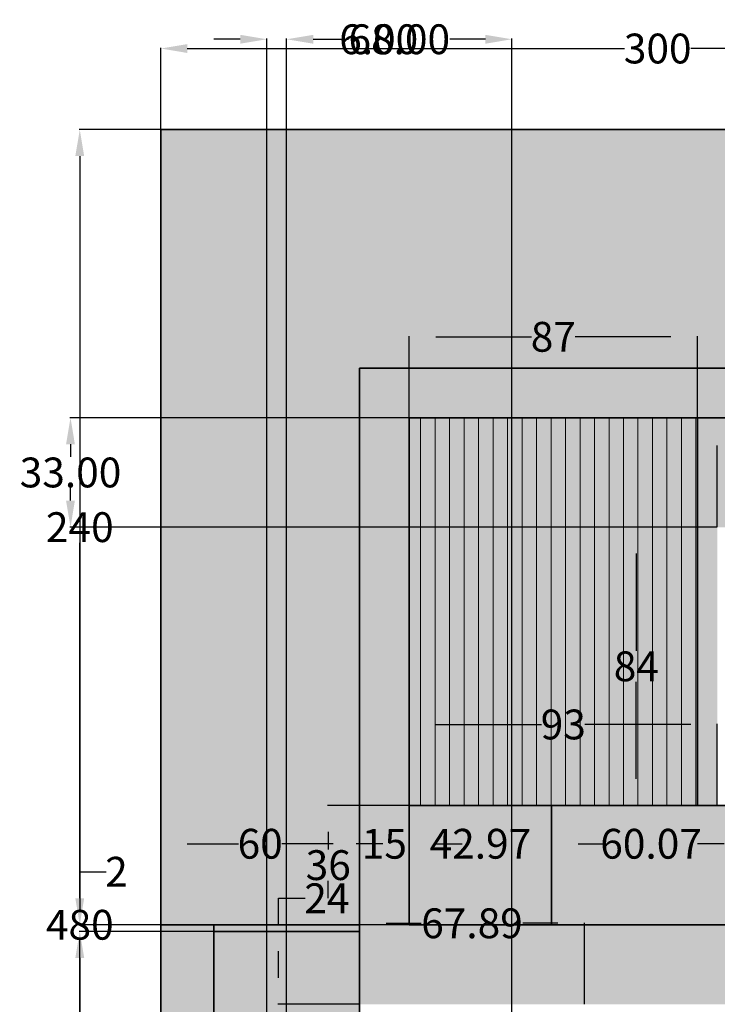
# Model space of a CAD drawing. Units: inches. Extents: x 207 to 609, y 30 to 576.
# Tile 3 of 4: x 207 to 418, y 279 to 576. Entities that reach past the tile are written whole.
import ezdxf

# ---------------------------------------------------------------- set-up
doc = ezdxf.new("R2010")
doc.units = ezdxf.units.IN
doc.header["$MEASUREMENT"] = 0
for name, color, linetype, lineweight in [('A-ANNO-DIMS', 2, 'Continuous', 18), ('A-ELEV', 7, 'Continuous', 35), ('A-ELEV-PATT', 251, 'Continuous', 13), ('A-ELEV-PATT-CLAD', 67, 'Continuous', 13), ('A-ELEV-PATT-WOOD', 19, 'Continuous', 13)]:
    doc.layers.add(name, color=color, linetype=linetype, lineweight=lineweight)
doc.styles.get("Standard").update_dxf_attribs({"font": 'arial.ttf'})
doc.dimstyles.get("Standard").update_dxf_attribs({"dimtxt": 9, "dimasz": 8, "dimexe": 0.18, "dimexo": 0.0625, "dimgap": 0.09, "dimtad": 0, "dimtih": 1, "dimtoh": 1, "dimdec": 0, "dimzin": 0, "dimdsep": 46, "dimlunit": 3, "dimtxsty": 'Standard', "dimcen": 0.09, "dimadec": 0, "dimazin": 0, "dimtfac": 1, "dimtdec": 0, "dimtofl": 0, "dimtmove": 0, "dimatfit": 3, "dimfxl": 1, "dimtolj": 1, "dimtzin": 0, "dimarcsym": 0})

# ---------------------------------------------------------------- blocks, each defined once
blk = doc.blocks.new('*D7')
at = {"layer": 'A-ANNO-DIMS', "color": 0, "lineweight": -2, "transparency": 16777216}
for p, q in [((249.7, 542.85), (249.7, 567.42)), ((257.7, 567.24), (389.68, 567.24)), ((541.7, 567.24), (409.71, 567.24)), ((549.7, 542.85), (549.7, 567.42))]:
    blk.add_line(p, q, dxfattribs=at)
at = {"layer": 'A-ANNO-DIMS', "color": 0, "transparency": 16777216}
for points in [[(257.7, 568.57), (257.7, 565.9), (249.7, 567.24)], [(541.7, 568.57), (541.7, 565.9), (549.7, 567.24)]]:
    blk.add_solid(points, dxfattribs=at)
at = {"layer": 'Defpoints', "color": 0, "transparency": 16777216}
for p in [(549.7, 567.24), (249.7, 542.79), (549.7, 542.79)]:
    blk.add_point(p, dxfattribs=at)
at = {"layer": 'A-ANNO-DIMS', "color": 0, "transparency": 16777216, "insert": (399.7, 567.24), "char_height": 9, "attachment_point": 5}
blk.add_mtext('\\A1;300', dxfattribs=at)
blk = doc.blocks.new('*D8')
at = {"layer": 'A-ANNO-DIMS', "color": 0, "lineweight": -2, "transparency": 16777216}
for p, q in [((249.63, 542.79), (225.07, 542.79)), ((225.25, 534.79), (225.25, 307.47)), ((225.25, 70.79), (225.25, 298.1)), ((249.63, 62.79), (225.07, 62.79))]:
    blk.add_line(p, q, dxfattribs=at)
at = {"layer": 'A-ANNO-DIMS', "color": 0, "transparency": 16777216}
for points in [[(223.91, 534.79), (226.58, 534.79), (225.25, 542.79)], [(223.91, 70.79), (226.58, 70.79), (225.25, 62.79)]]:
    blk.add_solid(points, dxfattribs=at)
at = {"layer": 'Defpoints', "color": 0, "transparency": 16777216}
for p in [(225.25, 542.79), (249.7, 542.79), (249.7, 62.79)]:
    blk.add_point(p, dxfattribs=at)
at = {"layer": 'A-ANNO-DIMS', "color": 0, "transparency": 16777216, "insert": (225.25, 302.79), "char_height": 9, "attachment_point": 5}
blk.add_mtext('\\A1;480', dxfattribs=at)
blk = doc.blocks.new('*D15')
at = {"layer": 'A-ANNO-DIMS', "color": 0, "lineweight": -2, "transparency": 16777216}
for p, q in [((265.63, 300.79), (225.07, 300.79)), ((225.25, 292.79), (225.25, 270.47)), ((225.25, 238.79), (225.25, 261.1)), ((265.63, 230.79), (225.07, 230.79))]:
    blk.add_line(p, q, dxfattribs=at)
at = {"layer": 'A-ANNO-DIMS', "color": 0, "transparency": 16777216}
for points in [[(223.91, 292.79), (226.58, 292.79), (225.25, 300.79)], [(223.91, 238.79), (226.58, 238.79), (225.25, 230.79)]]:
    blk.add_solid(points, dxfattribs=at)
at = {"layer": 'Defpoints', "color": 0, "transparency": 16777216}
for p in [(225.25, 300.79), (265.7, 300.79), (265.7, 230.79)]:
    blk.add_point(p, dxfattribs=at)
at = {"layer": 'A-ANNO-DIMS', "color": 0, "transparency": 16777216, "insert": (225.25, 265.79), "char_height": 9, "attachment_point": 5}
blk.add_mtext('\\A1;70', dxfattribs=at)
blk = doc.blocks.new('*D16')
at = {"layer": 'A-ANNO-DIMS', "color": 0, "lineweight": -2, "transparency": 16777216}
for p, q in [((225.25, 310.79), (225.25, 318.79)), ((225.25, 318.79), (233.25, 318.79)), ((265.63, 302.79), (225.07, 302.79)), ((265.63, 300.79), (225.07, 300.79)), ((225.25, 292.79), (225.25, 284.79))]:
    blk.add_line(p, q, dxfattribs=at)
at = {"layer": 'A-ANNO-DIMS', "color": 0, "transparency": 16777216}
for points in [[(223.91, 310.79), (226.58, 310.79), (225.25, 302.79)], [(223.91, 292.79), (226.58, 292.79), (225.25, 300.79)]]:
    blk.add_solid(points, dxfattribs=at)
at = {"layer": 'Defpoints', "color": 0, "transparency": 16777216}
for p in [(225.25, 302.79), (265.7, 302.79), (265.7, 300.79)]:
    blk.add_point(p, dxfattribs=at)
at = {"layer": 'A-ANNO-DIMS', "color": 0, "transparency": 16777216, "insert": (236.32, 318.79), "char_height": 9, "attachment_point": 5}
blk.add_mtext('\\A1;2', dxfattribs=at)
blk = doc.blocks.new('*D17')
at = {"layer": 'A-ANNO-DIMS', "color": 0, "lineweight": -2, "transparency": 16777216}
for p, q in [((249.63, 542.79), (225.07, 542.79)), ((225.25, 534.79), (225.25, 427.47)), ((225.25, 310.79), (225.25, 418.1)), ((249.63, 302.79), (225.07, 302.79))]:
    blk.add_line(p, q, dxfattribs=at)
at = {"layer": 'A-ANNO-DIMS', "color": 0, "transparency": 16777216}
for points in [[(223.91, 534.79), (226.58, 534.79), (225.25, 542.79)], [(223.91, 310.79), (226.58, 310.79), (225.25, 302.79)]]:
    blk.add_solid(points, dxfattribs=at)
at = {"layer": 'Defpoints', "color": 0, "transparency": 16777216}
for p in [(225.25, 542.79), (249.7, 542.79), (249.7, 302.79)]:
    blk.add_point(p, dxfattribs=at)
at = {"layer": 'A-ANNO-DIMS', "color": 0, "transparency": 16777216, "insert": (225.25, 422.79), "char_height": 9, "attachment_point": 5}
blk.add_mtext('\\A1;240', dxfattribs=at)
blk = doc.blocks.new('*D26')
at = {"layer": 'A-ANNO-DIMS', "color": 0, "lineweight": -2, "transparency": 16777216}
for p, q in [((285.25, 302.79), (285.25, 310.79)), ((285.25, 310.79), (293.25, 310.79)), ((309.63, 302.79), (285.07, 302.79)), ((285.25, 286.79), (285.25, 294.79)), ((309.63, 278.79), (285.07, 278.79))]:
    blk.add_line(p, q, dxfattribs=at)
at = {"layer": 'A-ANNO-DIMS', "color": 0, "transparency": 16777216}
for points in [[(283.91, 294.79), (286.58, 294.79), (285.25, 302.79)], [(283.91, 286.79), (286.58, 286.79), (285.25, 278.79)]]:
    blk.add_solid(points, dxfattribs=at)
at = {"layer": 'Defpoints', "color": 0, "transparency": 16777216}
for p in [(285.25, 302.79), (309.7, 302.79), (309.7, 278.79)]:
    blk.add_point(p, dxfattribs=at)
at = {"layer": 'A-ANNO-DIMS', "color": 0, "transparency": 16777216, "insert": (299.84, 310.79), "char_height": 9, "attachment_point": 5}
blk.add_mtext('\\A1;24', dxfattribs=at)
blk = doc.blocks.new('*D39')
at = {"layer": 'A-ANNO-DIMS', "color": 0, "lineweight": -2, "transparency": 16777216}
for p, q in [((249.7, 302.85), (249.7, 327.42)), ((257.7, 327.24), (273.15, 327.24)), ((301.7, 327.24), (286.24, 327.24)), ((309.7, 302.85), (309.7, 327.42))]:
    blk.add_line(p, q, dxfattribs=at)
at = {"layer": 'A-ANNO-DIMS', "color": 0, "transparency": 16777216}
for points in [[(257.7, 328.57), (257.7, 325.9), (249.7, 327.24)], [(301.7, 328.57), (301.7, 325.9), (309.7, 327.24)]]:
    blk.add_solid(points, dxfattribs=at)
at = {"layer": 'Defpoints', "color": 0, "transparency": 16777216}
for p in [(309.7, 327.24), (249.7, 302.79), (309.7, 302.79)]:
    blk.add_point(p, dxfattribs=at)
at = {"layer": 'A-ANNO-DIMS', "color": 0, "transparency": 16777216, "insert": (279.7, 327.24), "char_height": 9, "attachment_point": 5}
blk.add_mtext('\\A1;60', dxfattribs=at)
blk = doc.blocks.new('*D40')
at = {"layer": 'A-ANNO-DIMS', "color": 0, "lineweight": -2, "transparency": 16777216}
for p, q in [((301.7, 327.24), (293.7, 327.24)), ((309.7, 302.85), (309.7, 327.42)), ((324.7, 302.85), (324.7, 327.42)), ((332.7, 327.24), (340.7, 327.24))]:
    blk.add_line(p, q, dxfattribs=at)
at = {"layer": 'A-ANNO-DIMS', "color": 0, "transparency": 16777216}
for points in [[(301.7, 328.57), (301.7, 325.9), (309.7, 327.24)], [(332.7, 328.57), (332.7, 325.9), (324.7, 327.24)]]:
    blk.add_solid(points, dxfattribs=at)
at = {"layer": 'Defpoints', "color": 0, "transparency": 16777216}
for p in [(324.7, 327.24), (309.7, 302.79), (324.7, 302.79)]:
    blk.add_point(p, dxfattribs=at)
at = {"layer": 'A-ANNO-DIMS', "color": 0, "transparency": 16777216, "insert": (317.2, 327.24), "char_height": 9, "attachment_point": 5}
blk.add_mtext('\\A1;15', dxfattribs=at)
blk = doc.blocks.new('*D41')
at = {"layer": 'A-ANNO-DIMS', "color": 0, "lineweight": -2, "transparency": 16777216}
for p, q in [((324.7, 455.85), (324.7, 480.42)), ((332.7, 480.24), (361.65, 480.24)), ((403.7, 480.24), (374.74, 480.24)), ((411.7, 455.85), (411.7, 480.42))]:
    blk.add_line(p, q, dxfattribs=at)
at = {"layer": 'A-ANNO-DIMS', "color": 0, "transparency": 16777216}
for points in [[(332.7, 481.57), (332.7, 478.9), (324.7, 480.24)], [(403.7, 481.57), (403.7, 478.9), (411.7, 480.24)]]:
    blk.add_solid(points, dxfattribs=at)
at = {"layer": 'Defpoints', "color": 0, "transparency": 16777216}
for p in [(411.7, 480.24), (324.7, 455.79), (411.7, 455.79)]:
    blk.add_point(p, dxfattribs=at)
at = {"layer": 'A-ANNO-DIMS', "color": 0, "transparency": 16777216, "insert": (368.2, 480.24), "char_height": 9, "attachment_point": 5}
blk.add_mtext('\\A1;87', dxfattribs=at)
blk = doc.blocks.new('*D43')
at = {"layer": 'A-ANNO-DIMS', "color": 0, "lineweight": -2, "transparency": 16777216}
for p, q in [((324.7, 338.85), (324.7, 363.42)), ((332.7, 363.24), (364.66, 363.24)), ((409.7, 363.24), (377.73, 363.24)), ((417.7, 338.85), (417.7, 363.42))]:
    blk.add_line(p, q, dxfattribs=at)
at = {"layer": 'A-ANNO-DIMS', "color": 0, "transparency": 16777216}
for points in [[(332.7, 364.57), (332.7, 361.9), (324.7, 363.24)], [(409.7, 364.57), (409.7, 361.9), (417.7, 363.24)]]:
    blk.add_solid(points, dxfattribs=at)
at = {"layer": 'Defpoints', "color": 0, "transparency": 16777216}
for p in [(417.7, 363.24), (324.7, 338.79), (417.7, 338.79)]:
    blk.add_point(p, dxfattribs=at)
at = {"layer": 'A-ANNO-DIMS', "color": 0, "transparency": 16777216, "insert": (371.2, 363.24), "char_height": 9, "attachment_point": 5}
blk.add_mtext('\\A1;93', dxfattribs=at)
blk = doc.blocks.new('*D44')
at = {"layer": 'A-ANNO-DIMS', "color": 0, "lineweight": -2, "transparency": 16777216}
for p, q in [((417.7, 422.85), (417.7, 447.42)), ((425.7, 447.24), (438.18, 447.24)), ((463.7, 447.24), (451.21, 447.24)), ((471.7, 422.85), (471.7, 447.42))]:
    blk.add_line(p, q, dxfattribs=at)
at = {"layer": 'A-ANNO-DIMS', "color": 0, "transparency": 16777216}
for points in [[(425.7, 448.57), (425.7, 445.9), (417.7, 447.24)], [(463.7, 448.57), (463.7, 445.9), (471.7, 447.24)]]:
    blk.add_solid(points, dxfattribs=at)
at = {"layer": 'Defpoints', "color": 0, "transparency": 16777216}
for p in [(471.7, 447.24), (417.7, 422.79), (471.7, 422.79)]:
    blk.add_point(p, dxfattribs=at)
at = {"layer": 'A-ANNO-DIMS', "color": 0, "transparency": 16777216, "insert": (444.7, 447.24), "char_height": 9, "attachment_point": 5}
blk.add_mtext('\\A1;54', dxfattribs=at)
blk = doc.blocks.new('*D47')
at = {"layer": 'A-ANNO-DIMS', "color": 0, "lineweight": -2, "transparency": 16777216}
for p, q in [((316.7, 327.24), (308.7, 327.24)), ((324.7, 302.85), (324.7, 327.42)), ((367.66, 302.85), (367.66, 327.42)), ((375.66, 327.24), (383.66, 327.24))]:
    blk.add_line(p, q, dxfattribs=at)
at = {"layer": 'A-ANNO-DIMS', "color": 0, "transparency": 16777216}
for points in [[(316.7, 328.57), (316.7, 325.9), (324.7, 327.24)], [(375.66, 328.57), (375.66, 325.9), (367.66, 327.24)]]:
    blk.add_solid(points, dxfattribs=at)
at = {"layer": 'Defpoints', "color": 0, "transparency": 16777216}
for p in [(367.66, 327.24), (324.7, 302.79), (367.66, 302.79)]:
    blk.add_point(p, dxfattribs=at)
at = {"layer": 'A-ANNO-DIMS', "color": 0, "transparency": 16777216, "insert": (346.18, 327.24), "char_height": 9, "attachment_point": 5}
blk.add_mtext('\\A1;42.97', dxfattribs=at)
blk = doc.blocks.new('*D48')
at = {"layer": 'A-ANNO-DIMS', "color": 0, "lineweight": -2, "transparency": 16777216}
for p, q in [((367.66, 302.85), (367.66, 327.42)), ((375.66, 327.24), (382.4, 327.24)), ((419.73, 327.24), (413, 327.24)), ((427.73, 302.85), (427.73, 327.42))]:
    blk.add_line(p, q, dxfattribs=at)
at = {"layer": 'A-ANNO-DIMS', "color": 0, "transparency": 16777216}
for points in [[(375.66, 328.57), (375.66, 325.9), (367.66, 327.24)], [(419.73, 328.57), (419.73, 325.9), (427.73, 327.24)]]:
    blk.add_solid(points, dxfattribs=at)
at = {"layer": 'Defpoints', "color": 0, "transparency": 16777216}
for p in [(427.73, 327.24), (367.66, 302.79), (427.73, 302.79)]:
    blk.add_point(p, dxfattribs=at)
at = {"layer": 'A-ANNO-DIMS', "color": 0, "transparency": 16777216, "insert": (397.7, 327.24), "char_height": 9, "attachment_point": 5}
blk.add_mtext('\\A1;60.07', dxfattribs=at)
blk = doc.blocks.new('*D49')
at = {"layer": 'A-ANNO-DIMS', "color": 0, "lineweight": -2, "transparency": 16777216}
for p, q in [((419.73, 327.24), (411.73, 327.24)), ((427.73, 302.85), (427.73, 327.42)), ((459.05, 302.85), (459.05, 327.42)), ((467.05, 327.24), (475.05, 327.24))]:
    blk.add_line(p, q, dxfattribs=at)
at = {"layer": 'A-ANNO-DIMS', "color": 0, "transparency": 16777216}
for points in [[(419.73, 328.57), (419.73, 325.9), (427.73, 327.24)], [(467.05, 328.57), (467.05, 325.9), (459.05, 327.24)]]:
    blk.add_solid(points, dxfattribs=at)
at = {"layer": 'Defpoints', "color": 0, "transparency": 16777216}
for p in [(459.05, 327.24), (427.73, 302.79), (459.05, 302.79)]:
    blk.add_point(p, dxfattribs=at)
at = {"layer": 'A-ANNO-DIMS', "color": 0, "transparency": 16777216, "insert": (443.39, 327.24), "char_height": 9, "attachment_point": 5}
blk.add_mtext('\\A1;31.32', dxfattribs=at)
blk = doc.blocks.new('*D51')
at = {"layer": 'A-ANNO-DIMS', "color": 0, "lineweight": -2, "transparency": 16777216}
for p, q in [((324.63, 338.79), (300.07, 338.79)), ((300.25, 330.79), (300.25, 325.47)), ((300.25, 310.79), (300.25, 316.1)), ((324.63, 302.79), (300.07, 302.79))]:
    blk.add_line(p, q, dxfattribs=at)
at = {"layer": 'A-ANNO-DIMS', "color": 0, "transparency": 16777216}
for points in [[(298.91, 330.79), (301.58, 330.79), (300.25, 338.79)], [(298.91, 310.79), (301.58, 310.79), (300.25, 302.79)]]:
    blk.add_solid(points, dxfattribs=at)
at = {"layer": 'Defpoints', "color": 0, "transparency": 16777216}
for p in [(300.25, 338.79), (324.7, 338.79), (324.7, 302.79)]:
    blk.add_point(p, dxfattribs=at)
at = {"layer": 'A-ANNO-DIMS', "color": 0, "transparency": 16777216, "insert": (300.25, 320.79), "char_height": 9, "attachment_point": 5}
blk.add_mtext('\\A1;36', dxfattribs=at)
blk = doc.blocks.new('*D52')
at = {"layer": 'A-ANNO-DIMS', "color": 0, "lineweight": -2, "transparency": 16777216}
for p, q in [((417.63, 422.79), (393.07, 422.79)), ((393.25, 414.79), (393.25, 385.47)), ((393.25, 346.79), (393.25, 376.1)), ((417.63, 338.79), (393.07, 338.79))]:
    blk.add_line(p, q, dxfattribs=at)
at = {"layer": 'A-ANNO-DIMS', "color": 0, "transparency": 16777216}
for points in [[(391.91, 414.79), (394.58, 414.79), (393.25, 422.79)], [(391.91, 346.79), (394.58, 346.79), (393.25, 338.79)]]:
    blk.add_solid(points, dxfattribs=at)
at = {"layer": 'Defpoints', "color": 0, "transparency": 16777216}
for p in [(393.25, 422.79), (417.7, 422.79), (417.7, 338.79)]:
    blk.add_point(p, dxfattribs=at)
at = {"layer": 'A-ANNO-DIMS', "color": 0, "transparency": 16777216, "insert": (393.25, 380.79), "char_height": 9, "attachment_point": 5}
blk.add_mtext('\\A1;84', dxfattribs=at)
blk = doc.blocks.new('*D60')
at = {"layer": 'A-ANNO-DIMS', "color": 0, "lineweight": -2, "transparency": 16777216}
for p, q in [((309.7, 278.85), (309.7, 303.42)), ((317.7, 303.24), (328.33, 303.24)), ((369.58, 303.24), (358.95, 303.24)), ((377.58, 278.85), (377.58, 303.42))]:
    blk.add_line(p, q, dxfattribs=at)
at = {"layer": 'A-ANNO-DIMS', "color": 0, "transparency": 16777216}
for points in [[(317.7, 304.57), (317.7, 301.9), (309.7, 303.24)], [(369.58, 304.57), (369.58, 301.9), (377.58, 303.24)]]:
    blk.add_solid(points, dxfattribs=at)
at = {"layer": 'Defpoints', "color": 0, "transparency": 16777216}
for p in [(377.58, 303.24), (309.7, 278.79), (377.58, 278.79)]:
    blk.add_point(p, dxfattribs=at)
at = {"layer": 'A-ANNO-DIMS', "color": 0, "transparency": 16777216, "insert": (343.64, 303.24), "char_height": 9, "attachment_point": 5}
blk.add_mtext('\\A1;67.89', dxfattribs=at)
blk = doc.blocks.new('*D71')
at = {"layer": 'A-ANNO-DIMS', "color": 0, "lineweight": -2, "transparency": 16777216}
for p, q in [((273.7, 570.04), (265.7, 570.04)), ((281.7, 202.85), (281.7, 570.22)), ((287.7, 196.85), (287.7, 570.22)), ((295.7, 570.04), (303.7, 570.04))]:
    blk.add_line(p, q, dxfattribs=at)
at = {"layer": 'A-ANNO-DIMS', "color": 0, "transparency": 16777216}
for points in [[(273.7, 571.37), (273.7, 568.7), (281.7, 570.04)], [(295.7, 571.37), (295.7, 568.7), (287.7, 570.04)]]:
    blk.add_solid(points, dxfattribs=at)
at = {"layer": 'Defpoints', "color": 0, "transparency": 16777216}
for p in [(287.7, 570.04), (281.7, 202.79), (287.7, 196.79)]:
    blk.add_point(p, dxfattribs=at)
at = {"layer": 'A-ANNO-DIMS', "color": 0, "transparency": 16777216, "insert": (315.48, 570.04), "char_height": 9, "attachment_point": 5}
blk.add_mtext('\\A1;6.00', dxfattribs=at)
blk = doc.blocks.new('*D72')
at = {"layer": 'A-ANNO-DIMS', "color": 0, "lineweight": -2, "transparency": 16777216}
for p, q in [((287.7, 196.85), (287.7, 570.22)), ((295.7, 570.04), (306.41, 570.04)), ((347.7, 570.04), (336.98, 570.04)), ((355.7, 196.85), (355.7, 570.22))]:
    blk.add_line(p, q, dxfattribs=at)
at = {"layer": 'A-ANNO-DIMS', "color": 0, "transparency": 16777216}
for points in [[(295.7, 571.37), (295.7, 568.7), (287.7, 570.04)], [(347.7, 571.37), (347.7, 568.7), (355.7, 570.04)]]:
    blk.add_solid(points, dxfattribs=at)
at = {"layer": 'Defpoints', "color": 0, "transparency": 16777216}
for p in [(355.7, 570.04), (287.7, 196.79), (355.7, 196.79)]:
    blk.add_point(p, dxfattribs=at)
at = {"layer": 'A-ANNO-DIMS', "color": 0, "transparency": 16777216, "insert": (321.7, 570.04), "char_height": 9, "attachment_point": 5}
blk.add_mtext('\\A1;68.00', dxfattribs=at)
blk = doc.blocks.new('*D78')
at = {"layer": 'A-ANNO-DIMS', "color": 0, "lineweight": -2, "transparency": 16777216}
for p, q in [((411.63, 455.79), (222.27, 455.79)), ((222.45, 447.79), (222.45, 443.97)), ((222.45, 430.79), (222.45, 434.6)), ((417.63, 422.79), (222.27, 422.79))]:
    blk.add_line(p, q, dxfattribs=at)
at = {"layer": 'A-ANNO-DIMS', "color": 0, "transparency": 16777216}
for points in [[(221.11, 447.79), (223.78, 447.79), (222.45, 455.79)], [(221.11, 430.79), (223.78, 430.79), (222.45, 422.79)]]:
    blk.add_solid(points, dxfattribs=at)
at = {"layer": 'Defpoints', "color": 0, "transparency": 16777216}
for p in [(222.45, 455.79), (411.7, 455.79), (417.7, 422.79)]:
    blk.add_point(p, dxfattribs=at)
at = {"layer": 'A-ANNO-DIMS', "color": 0, "transparency": 16777216, "insert": (222.45, 439.29), "char_height": 9, "attachment_point": 5}
blk.add_mtext('\\A1;33.00', dxfattribs=at)

msp = doc.modelspace()

# ---------------------------------------------------------------- hatches: boundary and pattern name
at = {"layer": 'A-ELEV-PATT'}
h = msp.add_hatch(color=256, dxfattribs=at)
h.dxf.hatch_style = 1
h.paths.add_polyline_path([(443.656, 542.7864), (249.6956, 542.7864), (249.6956, 302.7864), (309.6956, 302.7864), (309.6956, 470.7864), (443.656, 470.7864)])
h = msp.add_hatch(color=256, dxfattribs=at)
h.dxf.hatch_style = 1
h.paths.add_polyline_path([(549.6956, 470.7864), (309.6956, 470.7864), (309.6956, 278.7864), (549.6956, 278.7864), (549.6956, 302.7864), (324.6956, 302.7864), (324.6956, 455.7864), (549.6956, 455.7864)])
h = msp.add_hatch(color=256, dxfattribs=at)
h.dxf.hatch_style = 1
h.paths.add_polyline_path([(477.6956, 455.7864), (411.6956, 455.7864), (411.6956, 338.7864), (417.6956, 338.7864), (417.6956, 422.7864), (471.6956, 422.7864), (471.6956, 338.7864), (477.6956, 338.7864)])
at = {"layer": 'A-ELEV-PATT', "transparency": 33554656}
h = msp.add_hatch(color=256, dxfattribs=at)
h.paths.add_polyline_path([(367.6635, 338.7864), (324.6956, 338.7864), (324.6956, 302.7864), (367.6635, 302.7864)])
h.paths.add_polyline_path([(427.7296, 338.7864), (367.6635, 338.7864), (367.6635, 302.7864), (427.7296, 302.7864)])
h.paths.add_polyline_path([(459.0525, 338.7864), (427.7296, 338.7864), (427.7296, 302.7864), (459.0525, 302.7864)])
h.paths.add_polyline_path([(477.6956, 338.7864), (459.0525, 338.7864), (459.0525, 302.7864), (477.6956, 302.7864)])
at = {"layer": 'A-ELEV-PATT'}
h = msp.add_hatch(color=256, dxfattribs=at)
h.dxf.hatch_style = 1
h.paths.add_polyline_path([(265.6956, 302.7864), (249.6956, 302.7864), (249.6956, 230.7864), (265.6956, 230.7864)])
h.paths.add_polyline_path([(265.6956, 218.7864), (249.6956, 218.7864), (249.6956, 62.7864), (265.6956, 62.7864)])
h.paths.add_polyline_path([(549.6956, 278.7864), (443.5808, 278.7864), (443.5808, 230.7864), (549.6956, 230.7864)])
h.paths.add_polyline_path([(534.6005, 237.2568), (450.425, 237.2568), (450.425, 269.6636), (534.6005, 269.6636)], flags=16)
h.paths.add_polyline_path([(531.6005, 240.2568), (453.425, 240.2568), (453.425, 266.6636), (531.6005, 266.6636)], flags=0)
at = {"layer": 'A-ELEV-PATT', "transparency": 33554656}
h = msp.add_hatch(color=256, dxfattribs=at)
h.set_gradient(color1=(215, 235, 210), color2=(99, 100, 102), rotation=180)
h.paths.add_polyline_path([(265.6956, 230.7864), (309.6956, 230.7864), (309.6956, 300.7864), (265.6956, 300.7864)])
at = {"layer": 'A-ELEV-PATT-CLAD', "transparency": 33554656}
h = msp.add_hatch(dxfattribs=at)
h.set_pattern_fill('ANSI31', color=256, scale=35, angle=45, style=0)
h.paths.add_polyline_path([(411.6956, 455.7864), (324.6956, 455.7864), (324.6956, 338.7864), (411.6956, 338.7864)])
at = {"layer": 'A-ELEV-PATT-WOOD', "transparency": 33554656}
for points in [[(411.6956, 455.7864), (324.6956, 455.7864), (324.6956, 338.7864), (411.6956, 338.7864)], [(309.6956, 302.7864), (265.6956, 302.7864), (265.6956, 300.7864), (309.6956, 300.7864)]]:
    msp.add_hatch(color=256, dxfattribs=at).paths.add_polyline_path(points)

# ---------------------------------------------------------------- linework, layer by layer
at = {"layer": 'A-ELEV'}
for p, q in [((249.6956, 542.7864), (549.6956, 542.7864)), ((249.6956, 542.7864), (249.6956, 62.7864)), ((309.6956, 470.7864), (309.6956, 230.7864)), ((309.6956, 470.7864), (549.6956, 470.7864)), ((324.6956, 455.7864), (549.6956, 455.7864)), ((324.6956, 455.7864), (324.6956, 302.7864)), ((411.6956, 455.7864), (411.6956, 338.7864)), ((477.6956, 338.7864), (324.6956, 338.7864)), ((367.6635, 338.7864), (367.6635, 302.7864)), ((309.6956, 302.7864), (249.6956, 302.7864)), ((265.6956, 302.7864), (265.6956, 230.7864)), ((309.6956, 300.7864), (265.6956, 300.7864)), ((549.6956, 302.7864), (324.6956, 302.7864))]:
    msp.add_line(p, q, dxfattribs=at)

# ---------------------------------------------------------------- dimensions: what is measured, and where the dimension line sits
at = {"layer": 'A-ANNO-DIMS'}
for base, p1, p2, override, picture, middle in [((287.6956, 570.0364), (281.6956, 202.7864), (287.6956, 196.7864), {"dimdec": 2, "dimlfac": 1, "dimrnd": 0, "dimzin": 0, "dimdsep": 46, "dimlunit": 2}, '*D71', (315.4837, 570.0364)), ((355.6956, 570.0364), (287.6956, 196.7864), (355.6956, 196.7864), {"dimdec": 2, "dimlfac": 1, "dimrnd": 0, "dimzin": 0, "dimdsep": 46, "dimlunit": 2}, '*D72', (321.6956, 570.0364)), ((549.6956, 567.2364), (249.6956, 542.7864), (549.6956, 542.7864), {"dimdec": 0, "dimlfac": 1, "dimrnd": 0, "dimzin": 0, "dimdsep": 46, "dimlunit": 2}, '*D7', (399.6956, 567.2364)), ((411.6956, 480.2364), (324.6956, 455.7864), (411.6956, 455.7864), {"dimdec": 0, "dimlfac": 1, "dimrnd": 0, "dimzin": 0, "dimdsep": 46, "dimlunit": 2}, '*D41', (368.1956, 480.2364)), ((471.6956, 447.2364), (417.6956, 422.7864), (471.6956, 422.7864), {"dimdec": 0, "dimlfac": 1, "dimrnd": 0, "dimzin": 0, "dimdsep": 46, "dimlunit": 2}, '*D44', (444.6956, 447.2364)), ((417.6956, 363.2364), (324.6956, 338.7864), (417.6956, 338.7864), {"dimdec": 0, "dimlfac": 1, "dimrnd": 0, "dimzin": 0, "dimdsep": 46, "dimlunit": 2}, '*D43', (371.1956, 363.2364)), ((309.6956, 327.2364), (249.6956, 302.7864), (309.6956, 302.7864), {"dimdec": 0, "dimlfac": 1, "dimrnd": 0, "dimzin": 0, "dimdsep": 46, "dimlunit": 2}, '*D39', (279.6956, 327.2364)), ((324.6956, 327.2364), (309.6956, 302.7864), (324.6956, 302.7864), {"dimdec": 0, "dimlfac": 1, "dimrnd": 0, "dimzin": 0, "dimdsep": 46, "dimlunit": 2}, '*D40', (317.1956, 327.2364)), ((367.6635, 327.2364), (324.6956, 302.7864), (367.6635, 302.7864), {"dimdec": 2, "dimlfac": 1, "dimrnd": 0, "dimzin": 0, "dimdsep": 46, "dimlunit": 2}, '*D47', (346.1795, 327.2364)), ((427.7296, 327.2364), (367.6635, 302.7864), (427.7296, 302.7864), {"dimdec": 2, "dimlfac": 1, "dimrnd": 0, "dimzin": 0, "dimdsep": 46, "dimlunit": 2}, '*D48', (397.6965, 327.2364)), ((459.0525, 327.2364), (427.7296, 302.7864), (459.0525, 302.7864), {"dimdec": 2, "dimlfac": 1, "dimrnd": 0, "dimzin": 0, "dimdsep": 46, "dimlunit": 2}, '*D49', (443.3911, 327.2364)), ((377.5808, 303.2364), (309.6956, 278.7864), (377.5808, 278.7864), {"dimdec": 2, "dimlfac": 1, "dimrnd": 0, "dimzin": 0, "dimdsep": 46, "dimlunit": 2}, '*D60', (343.6382, 303.2364))]:
    dim = msp.add_linear_dim(base=base, p1=p1, p2=p2, dimstyle='Standard', override=override, dxfattribs=at)
    dim.commit()
    dim.dimension.update_dxf_attribs({"geometry": picture, "text_midpoint": middle})
for base, p1, p2, override, picture, middle in [((225.2456, 542.7864), (249.6956, 62.7864), (249.6956, 542.7864), {"dimdec": 0, "dimlfac": 1, "dimrnd": 0, "dimzin": 0, "dimdsep": 46, "dimlunit": 2}, '*D8', (225.2456, 302.7864)), ((225.2456, 542.7864), (249.6956, 302.7864), (249.6956, 542.7864), {"dimdec": 0, "dimlfac": 1, "dimrnd": 0, "dimzin": 0, "dimdsep": 46, "dimlunit": 2}, '*D17', (225.2456, 422.7864)), ((222.4456, 455.7864), (417.6956, 422.7864), (411.6956, 455.7864), {"dimdec": 2, "dimlfac": 1, "dimrnd": 0, "dimzin": 0, "dimdsep": 46, "dimlunit": 2}, '*D78', (222.4456, 439.2864)), ((393.2456, 422.7864), (417.6956, 338.7864), (417.6956, 422.7864), {"dimdec": 0, "dimlfac": 1, "dimrnd": 0, "dimzin": 0, "dimdsep": 46, "dimlunit": 2}, '*D52', (393.2456, 380.7864)), ((300.2456, 338.7864), (324.6956, 302.7864), (324.6956, 338.7864), {"dimdec": 0, "dimlfac": 1, "dimrnd": 0, "dimzin": 0, "dimdsep": 46, "dimlunit": 2}, '*D51', (300.2456, 320.7864)), ((225.2456, 302.7864), (265.6956, 300.7864), (265.6956, 302.7864), {"dimdec": 0, "dimlfac": 1, "dimrnd": 0, "dimzin": 0, "dimdsep": 46, "dimlunit": 2}, '*D16', (236.3161, 318.7864)), ((285.2456, 302.7864), (309.6956, 278.7864), (309.6956, 302.7864), {"dimdec": 0, "dimlfac": 1, "dimrnd": 0, "dimzin": 0, "dimdsep": 46, "dimlunit": 2}, '*D26', (299.84, 310.7864)), ((225.2456, 300.7864), (265.6956, 230.7864), (265.6956, 300.7864), {"dimdec": 0, "dimlfac": 1, "dimrnd": 0, "dimzin": 0, "dimdsep": 46, "dimlunit": 2}, '*D15', (225.2456, 265.7864))]:
    dim = msp.add_linear_dim(base=base, p1=p1, p2=p2, angle=90, dimstyle='Standard', override=override, dxfattribs=at)
    dim.commit()
    dim.dimension.update_dxf_attribs({"geometry": picture, "text_midpoint": middle})

doc.saveas('drawing.dxf')
